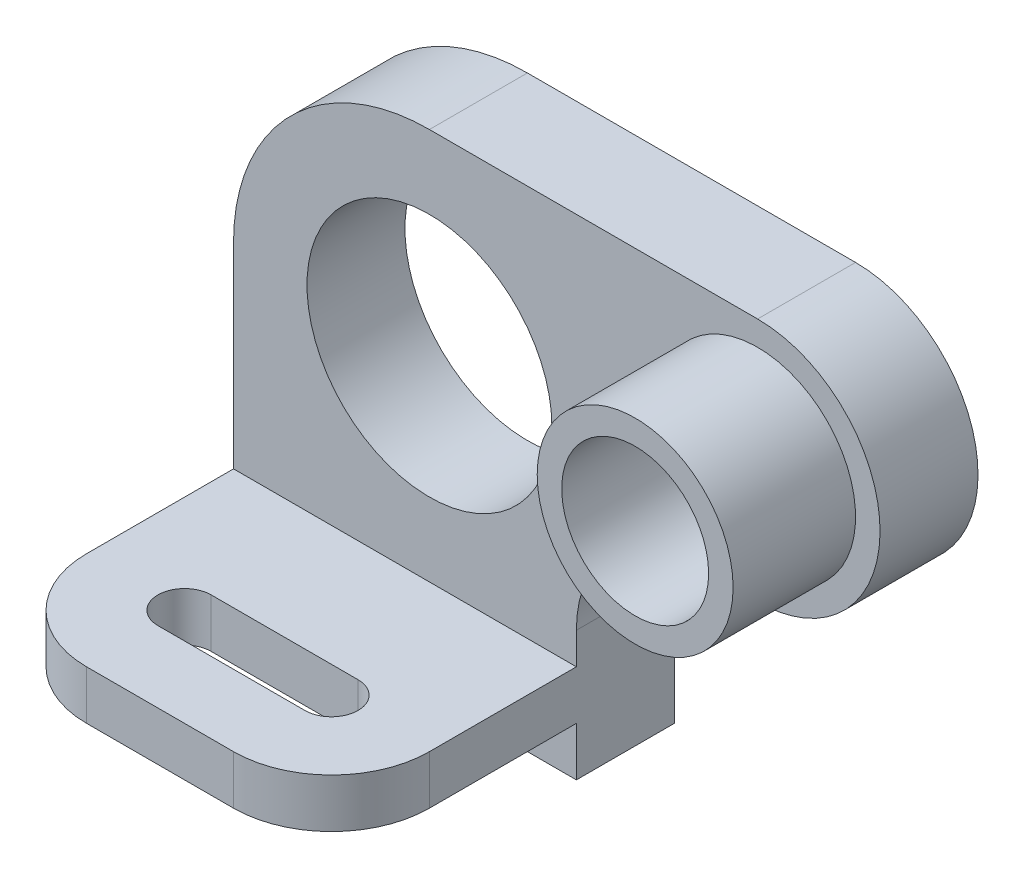
ISO-10303-21;
HEADER;
FILE_DESCRIPTION(('STEP AP214'),'2;1');
FILE_NAME('part.step','',(''),(''),'','','');
FILE_SCHEMA(('AUTOMOTIVE_DESIGN { 1 0 10303 214 1 1 1 1 }'));
ENDSEC;
DATA;
#1=APPLICATION_CONTEXT('core data for automotive mechanical design processes');
#2=APPLICATION_PROTOCOL_DEFINITION('international standard','automotive_design',2000,#1);
#3=PRODUCT_CONTEXT('',#1,'mechanical');
#4=PRODUCT('Part','Part','',(#3));
#5=PRODUCT_RELATED_PRODUCT_CATEGORY('part','',(#4));
#6=PRODUCT_DEFINITION_FORMATION('','',#4);
#7=PRODUCT_DEFINITION_CONTEXT('part definition',#1,'design');
#8=PRODUCT_DEFINITION('design','',#6,#7);
#9=PRODUCT_DEFINITION_SHAPE('','',#8);
#10=(LENGTH_UNIT() NAMED_UNIT(*) SI_UNIT(.MILLI.,.METRE.));
#11=(NAMED_UNIT(*) PLANE_ANGLE_UNIT() SI_UNIT($,.RADIAN.));
#12=(NAMED_UNIT(*) SI_UNIT($,.STERADIAN.) SOLID_ANGLE_UNIT());
#13=UNCERTAINTY_MEASURE_WITH_UNIT(LENGTH_MEASURE(1.E-05),#10,'distance_accuracy_value','');
#14=(GEOMETRIC_REPRESENTATION_CONTEXT(3) GLOBAL_UNCERTAINTY_ASSIGNED_CONTEXT((#13)) GLOBAL_UNIT_ASSIGNED_CONTEXT((#10,
#11,#12)) REPRESENTATION_CONTEXT('',''));
#15=CARTESIAN_POINT('',(0.,0.,0.));
#16=DIRECTION('',(0.,0.,1.));
#17=DIRECTION('',(1.,0.,0.));
#18=AXIS2_PLACEMENT_3D('',#15,#16,#17);
#19=CARTESIAN_POINT('',(40.,60.,20.));
#20=DIRECTION('',(0.,0.,-1.));
#21=DIRECTION('',(-1.,0.,0.));
#22=AXIS2_PLACEMENT_3D('',#19,#20,#21);
#23=PLANE('',#22);
#24=CARTESIAN_POINT('',(107.,75.,20.));
#25=DIRECTION('',(0.,0.,-1.));
#26=DIRECTION('',(-1.,0.,0.));
#27=AXIS2_PLACEMENT_3D('',#24,#25,#26);
#28=CIRCLE('',#27,20.);
#29=CARTESIAN_POINT('',(87.,75.,20.));
#30=VERTEX_POINT('',#29);
#31=EDGE_CURVE('E281',#30,#30,#28,.F.);
#32=ORIENTED_EDGE('',*,*,#31,.F.);
#33=EDGE_LOOP('',(#32));
#34=FACE_BOUND('',#33,.T.);
#35=CARTESIAN_POINT('',(40.,60.,20.));
#36=DIRECTION('',(0.,0.,1.));
#37=DIRECTION('',(1.,0.,0.));
#38=AXIS2_PLACEMENT_3D('',#35,#36,#37);
#39=CIRCLE('',#38,25.);
#40=CARTESIAN_POINT('',(65.,60.,20.));
#41=VERTEX_POINT('',#40);
#42=EDGE_CURVE('E215',#41,#41,#39,.T.);
#43=ORIENTED_EDGE('',*,*,#42,.F.);
#44=EDGE_LOOP('',(#43));
#45=FACE_BOUND('',#44,.T.);
#46=DIRECTION('',(-1.,0.,0.));
#47=VECTOR('',#46,1.);
#48=CARTESIAN_POINT('',(0.,20.,20.));
#49=LINE('',#48,#47);
#50=CARTESIAN_POINT('',(70.,20.,20.));
#51=VERTEX_POINT('',#50);
#52=CARTESIAN_POINT('',(0.,20.,20.));
#53=VERTEX_POINT('',#52);
#54=EDGE_CURVE('E190',#51,#53,#49,.T.);
#55=ORIENTED_EDGE('',*,*,#54,.F.);
#56=DIRECTION('',(0.,1.,0.));
#57=VECTOR('',#56,1.);
#58=CARTESIAN_POINT('',(70.,26.4613556019535,20.));
#59=LINE('',#58,#57);
#60=CARTESIAN_POINT('',(70.,26.4613556019535,20.));
#61=VERTEX_POINT('',#60);
#62=EDGE_CURVE('E232',#51,#61,#59,.T.);
#63=ORIENTED_EDGE('',*,*,#62,.T.);
#64=CARTESIAN_POINT('',(95.,26.4613556019535,20.));
#65=DIRECTION('',(0.,0.,-1.));
#66=DIRECTION('',(-1.,0.,0.));
#67=AXIS2_PLACEMENT_3D('',#64,#65,#66);
#68=CIRCLE('',#67,25.);
#69=CARTESIAN_POINT('',(101.,50.7306778009767,20.));
#70=VERTEX_POINT('',#69);
#71=EDGE_CURVE('E236',#61,#70,#68,.T.);
#72=ORIENTED_EDGE('',*,*,#71,.T.);
#73=CARTESIAN_POINT('',(107.,75.,20.));
#74=DIRECTION('',(0.,0.,1.));
#75=DIRECTION('',(1.,0.,0.));
#76=AXIS2_PLACEMENT_3D('',#73,#74,#75);
#77=CIRCLE('',#76,25.);
#78=CARTESIAN_POINT('',(107.,100.,20.));
#79=VERTEX_POINT('',#78);
#80=EDGE_CURVE('E238',#70,#79,#77,.T.);
#81=ORIENTED_EDGE('',*,*,#80,.T.);
#82=DIRECTION('',(-1.,0.,0.));
#83=VECTOR('',#82,1.);
#84=CARTESIAN_POINT('',(40.,100.,20.));
#85=LINE('',#84,#83);
#86=CARTESIAN_POINT('',(40.,100.,20.));
#87=VERTEX_POINT('',#86);
#88=EDGE_CURVE('E242',#79,#87,#85,.T.);
#89=ORIENTED_EDGE('',*,*,#88,.T.);
#90=CARTESIAN_POINT('',(40.,60.,20.));
#91=DIRECTION('',(0.,0.,1.));
#92=DIRECTION('',(-1.,0.,0.));
#93=AXIS2_PLACEMENT_3D('',#90,#91,#92);
#94=CIRCLE('',#93,40.);
#95=CARTESIAN_POINT('',(0.,60.,20.));
#96=VERTEX_POINT('',#95);
#97=EDGE_CURVE('E243',#87,#96,#94,.T.);
#98=ORIENTED_EDGE('',*,*,#97,.T.);
#99=DIRECTION('',(0.,-1.,0.));
#100=VECTOR('',#99,1.);
#101=CARTESIAN_POINT('',(0.,0.,20.));
#102=LINE('',#101,#100);
#103=EDGE_CURVE('E229',#96,#53,#102,.T.);
#104=ORIENTED_EDGE('',*,*,#103,.T.);
#105=EDGE_LOOP('',(#55,#63,#72,#81,#89,#98,#104));
#106=FACE_BOUND('',#105,.T.);
#107=ADVANCED_FACE('F44',(#34,#45,#106),#23,.F.);
#108=DIRECTION('',(1.,0.,0.));
#109=VECTOR('',#108,1.);
#110=CARTESIAN_POINT('',(0.,10.,20.));
#111=LINE('',#110,#109);
#112=CARTESIAN_POINT('',(0.,10.,20.));
#113=VERTEX_POINT('',#112);
#114=CARTESIAN_POINT('',(70.,10.,20.));
#115=VERTEX_POINT('',#114);
#116=EDGE_CURVE('E197',#113,#115,#111,.T.);
#117=ORIENTED_EDGE('',*,*,#116,.F.);
#118=CARTESIAN_POINT('',(0.,0.,20.));
#119=VERTEX_POINT('',#118);
#120=EDGE_CURVE('E235',#113,#119,#102,.T.);
#121=ORIENTED_EDGE('',*,*,#120,.T.);
#122=DIRECTION('',(1.,0.,0.));
#123=VECTOR('',#122,1.);
#124=CARTESIAN_POINT('',(0.,0.,20.));
#125=LINE('',#124,#123);
#126=CARTESIAN_POINT('',(70.,0.,20.));
#127=VERTEX_POINT('',#126);
#128=EDGE_CURVE('E231',#119,#127,#125,.T.);
#129=ORIENTED_EDGE('',*,*,#128,.T.);
#130=EDGE_CURVE('E234',#127,#115,#59,.T.);
#131=ORIENTED_EDGE('',*,*,#130,.T.);
#132=EDGE_LOOP('',(#117,#121,#129,#131));
#133=FACE_BOUND('',#132,.T.);
#134=ADVANCED_FACE('F324',(#133),#23,.F.);
#135=CARTESIAN_POINT('',(0.,0.,20.));
#136=DIRECTION('',(1.,0.,0.));
#137=DIRECTION('',(0.,0.,-1.));
#138=AXIS2_PLACEMENT_3D('',#135,#136,#137);
#139=PLANE('',#138);
#140=DIRECTION('',(0.,0.,-1.));
#141=VECTOR('',#140,1.);
#142=CARTESIAN_POINT('',(0.,10.,70.));
#143=LINE('',#142,#141);
#144=CARTESIAN_POINT('',(0.,10.,50.));
#145=VERTEX_POINT('',#144);
#146=EDGE_CURVE('E206',#145,#113,#143,.T.);
#147=ORIENTED_EDGE('',*,*,#146,.F.);
#148=DIRECTION('',(0.,-1.,0.));
#149=VECTOR('',#148,1.);
#150=CARTESIAN_POINT('',(0.,20.,50.));
#151=LINE('',#150,#149);
#152=CARTESIAN_POINT('',(0.,20.,50.));
#153=VERTEX_POINT('',#152);
#154=EDGE_CURVE('E294',#145,#153,#151,.F.);
#155=ORIENTED_EDGE('',*,*,#154,.T.);
#156=DIRECTION('',(0.,0.,-1.));
#157=VECTOR('',#156,1.);
#158=CARTESIAN_POINT('',(0.,20.,70.));
#159=LINE('',#158,#157);
#160=EDGE_CURVE('E208',#153,#53,#159,.T.);
#161=ORIENTED_EDGE('',*,*,#160,.T.);
#162=ORIENTED_EDGE('',*,*,#103,.F.);
#163=DIRECTION('',(0.,0.,-1.));
#164=VECTOR('',#163,1.);
#165=CARTESIAN_POINT('',(0.,60.,20.));
#166=LINE('',#165,#164);
#167=CARTESIAN_POINT('',(0.,60.,0.));
#168=VERTEX_POINT('',#167);
#169=EDGE_CURVE('E246',#96,#168,#166,.T.);
#170=ORIENTED_EDGE('',*,*,#169,.T.);
#171=DIRECTION('',(0.,-1.,0.));
#172=VECTOR('',#171,1.);
#173=CARTESIAN_POINT('',(0.,0.,0.));
#174=LINE('',#173,#172);
#175=CARTESIAN_POINT('',(0.,0.,0.));
#176=VERTEX_POINT('',#175);
#177=EDGE_CURVE('E227',#168,#176,#174,.T.);
#178=ORIENTED_EDGE('',*,*,#177,.T.);
#179=DIRECTION('',(0.,0.,-1.));
#180=VECTOR('',#179,1.);
#181=CARTESIAN_POINT('',(0.,0.,20.));
#182=LINE('',#181,#180);
#183=EDGE_CURVE('E279',#119,#176,#182,.T.);
#184=ORIENTED_EDGE('',*,*,#183,.F.);
#185=ORIENTED_EDGE('',*,*,#120,.F.);
#186=EDGE_LOOP('',(#147,#155,#161,#162,#170,#178,#184,#185));
#187=FACE_BOUND('',#186,.T.);
#188=ADVANCED_FACE('F335',(#187),#139,.F.);
#189=CARTESIAN_POINT('',(0.,0.,20.));
#190=DIRECTION('',(0.,1.,0.));
#191=DIRECTION('',(0.,0.,1.));
#192=AXIS2_PLACEMENT_3D('',#189,#190,#191);
#193=PLANE('',#192);
#194=DIRECTION('',(1.,0.,0.));
#195=VECTOR('',#194,1.);
#196=CARTESIAN_POINT('',(0.,0.,0.));
#197=LINE('',#196,#195);
#198=CARTESIAN_POINT('',(70.,0.,0.));
#199=VERTEX_POINT('',#198);
#200=EDGE_CURVE('E247',#176,#199,#197,.T.);
#201=ORIENTED_EDGE('',*,*,#200,.T.);
#202=DIRECTION('',(0.,0.,-1.));
#203=VECTOR('',#202,1.);
#204=CARTESIAN_POINT('',(70.,0.,20.));
#205=LINE('',#204,#203);
#206=EDGE_CURVE('E274',#127,#199,#205,.T.);
#207=ORIENTED_EDGE('',*,*,#206,.F.);
#208=ORIENTED_EDGE('',*,*,#128,.F.);
#209=ORIENTED_EDGE('',*,*,#183,.T.);
#210=EDGE_LOOP('',(#201,#207,#208,#209));
#211=FACE_BOUND('',#210,.T.);
#212=ADVANCED_FACE('F398',(#211),#193,.F.);
#213=CARTESIAN_POINT('',(70.,26.4613556019535,20.));
#214=DIRECTION('',(-1.,0.,0.));
#215=DIRECTION('',(0.,0.,1.));
#216=AXIS2_PLACEMENT_3D('',#213,#214,#215);
#217=PLANE('',#216);
#218=DIRECTION('',(0.,0.,-1.));
#219=VECTOR('',#218,1.);
#220=CARTESIAN_POINT('',(70.,20.,70.));
#221=LINE('',#220,#219);
#222=CARTESIAN_POINT('',(70.,20.,50.));
#223=VERTEX_POINT('',#222);
#224=EDGE_CURVE('E209',#223,#51,#221,.T.);
#225=ORIENTED_EDGE('',*,*,#224,.F.);
#226=DIRECTION('',(0.,1.,0.));
#227=VECTOR('',#226,1.);
#228=CARTESIAN_POINT('',(70.,10.,50.));
#229=LINE('',#228,#227);
#230=CARTESIAN_POINT('',(70.,10.,50.));
#231=VERTEX_POINT('',#230);
#232=EDGE_CURVE('E300',#223,#231,#229,.F.);
#233=ORIENTED_EDGE('',*,*,#232,.T.);
#234=DIRECTION('',(0.,0.,-1.));
#235=VECTOR('',#234,1.);
#236=CARTESIAN_POINT('',(70.,10.,70.));
#237=LINE('',#236,#235);
#238=EDGE_CURVE('E199',#231,#115,#237,.T.);
#239=ORIENTED_EDGE('',*,*,#238,.T.);
#240=ORIENTED_EDGE('',*,*,#130,.F.);
#241=ORIENTED_EDGE('',*,*,#206,.T.);
#242=DIRECTION('',(0.,1.,0.));
#243=VECTOR('',#242,1.);
#244=CARTESIAN_POINT('',(70.,26.4613556019535,0.));
#245=LINE('',#244,#243);
#246=CARTESIAN_POINT('',(70.,26.4613556019535,0.));
#247=VERTEX_POINT('',#246);
#248=EDGE_CURVE('E253',#199,#247,#245,.T.);
#249=ORIENTED_EDGE('',*,*,#248,.T.);
#250=DIRECTION('',(0.,0.,-1.));
#251=VECTOR('',#250,1.);
#252=CARTESIAN_POINT('',(70.,26.4613556019535,20.));
#253=LINE('',#252,#251);
#254=EDGE_CURVE('E275',#61,#247,#253,.T.);
#255=ORIENTED_EDGE('',*,*,#254,.F.);
#256=ORIENTED_EDGE('',*,*,#62,.F.);
#257=EDGE_LOOP('',(#225,#233,#239,#240,#241,#249,#255,#256));
#258=FACE_BOUND('',#257,.T.);
#259=ADVANCED_FACE('F393',(#258),#217,.F.);
#260=CARTESIAN_POINT('',(95.,26.4613556019535,20.));
#261=DIRECTION('',(0.,0.,-1.));
#262=DIRECTION('',(-1.,0.,0.));
#263=AXIS2_PLACEMENT_3D('',#260,#261,#262);
#264=CYLINDRICAL_SURFACE('',#263,25.);
#265=CARTESIAN_POINT('',(95.,26.4613556019535,0.));
#266=DIRECTION('',(0.,0.,-1.));
#267=DIRECTION('',(-1.,0.,0.));
#268=AXIS2_PLACEMENT_3D('',#265,#266,#267);
#269=CIRCLE('',#268,25.);
#270=CARTESIAN_POINT('',(101.,50.7306778009767,0.));
#271=VERTEX_POINT('',#270);
#272=EDGE_CURVE('E251',#247,#271,#269,.T.);
#273=ORIENTED_EDGE('',*,*,#272,.T.);
#274=DIRECTION('',(0.,0.,-1.));
#275=VECTOR('',#274,1.);
#276=CARTESIAN_POINT('',(101.,50.7306778009767,20.));
#277=LINE('',#276,#275);
#278=EDGE_CURVE('E267',#70,#271,#277,.T.);
#279=ORIENTED_EDGE('',*,*,#278,.F.);
#280=ORIENTED_EDGE('',*,*,#71,.F.);
#281=ORIENTED_EDGE('',*,*,#254,.T.);
#282=EDGE_LOOP('',(#273,#279,#280,#281));
#283=FACE_BOUND('',#282,.T.);
#284=ADVANCED_FACE('F388',(#283),#264,.F.);
#285=CARTESIAN_POINT('',(107.,75.,20.));
#286=DIRECTION('',(0.,0.,-1.));
#287=DIRECTION('',(-1.,0.,0.));
#288=AXIS2_PLACEMENT_3D('',#285,#286,#287);
#289=CYLINDRICAL_SURFACE('',#288,25.);
#290=CARTESIAN_POINT('',(107.,75.,0.));
#291=DIRECTION('',(0.,0.,1.));
#292=DIRECTION('',(1.,0.,0.));
#293=AXIS2_PLACEMENT_3D('',#290,#291,#292);
#294=CIRCLE('',#293,25.);
#295=CARTESIAN_POINT('',(107.,100.,0.));
#296=VERTEX_POINT('',#295);
#297=EDGE_CURVE('E254',#271,#296,#294,.T.);
#298=ORIENTED_EDGE('',*,*,#297,.T.);
#299=DIRECTION('',(0.,0.,-1.));
#300=VECTOR('',#299,1.);
#301=CARTESIAN_POINT('',(107.,100.,20.));
#302=LINE('',#301,#300);
#303=EDGE_CURVE('E266',#79,#296,#302,.T.);
#304=ORIENTED_EDGE('',*,*,#303,.F.);
#305=ORIENTED_EDGE('',*,*,#80,.F.);
#306=ORIENTED_EDGE('',*,*,#278,.T.);
#307=EDGE_LOOP('',(#298,#304,#305,#306));
#308=FACE_BOUND('',#307,.T.);
#309=ADVANCED_FACE('F387',(#308),#289,.T.);
#310=CARTESIAN_POINT('',(40.,100.,20.));
#311=DIRECTION('',(0.,-1.,0.));
#312=DIRECTION('',(1.,0.,0.));
#313=AXIS2_PLACEMENT_3D('',#310,#311,#312);
#314=PLANE('',#313);
#315=DIRECTION('',(-1.,0.,0.));
#316=VECTOR('',#315,1.);
#317=CARTESIAN_POINT('',(40.,100.,0.));
#318=LINE('',#317,#316);
#319=CARTESIAN_POINT('',(40.,100.,0.));
#320=VERTEX_POINT('',#319);
#321=EDGE_CURVE('E260',#296,#320,#318,.T.);
#322=ORIENTED_EDGE('',*,*,#321,.T.);
#323=DIRECTION('',(0.,0.,-1.));
#324=VECTOR('',#323,1.);
#325=CARTESIAN_POINT('',(40.,100.,20.));
#326=LINE('',#325,#324);
#327=EDGE_CURVE('E263',#87,#320,#326,.T.);
#328=ORIENTED_EDGE('',*,*,#327,.F.);
#329=ORIENTED_EDGE('',*,*,#88,.F.);
#330=ORIENTED_EDGE('',*,*,#303,.T.);
#331=EDGE_LOOP('',(#322,#328,#329,#330));
#332=FACE_BOUND('',#331,.T.);
#333=ADVANCED_FACE('F377',(#332),#314,.F.);
#334=CARTESIAN_POINT('',(40.,60.,20.));
#335=DIRECTION('',(0.,0.,-1.));
#336=DIRECTION('',(-1.,0.,0.));
#337=AXIS2_PLACEMENT_3D('',#334,#335,#336);
#338=CYLINDRICAL_SURFACE('',#337,40.);
#339=CARTESIAN_POINT('',(40.,60.,0.));
#340=DIRECTION('',(0.,0.,1.));
#341=DIRECTION('',(-1.,0.,0.));
#342=AXIS2_PLACEMENT_3D('',#339,#340,#341);
#343=CIRCLE('',#342,40.);
#344=EDGE_CURVE('E259',#320,#168,#343,.T.);
#345=ORIENTED_EDGE('',*,*,#344,.T.);
#346=ORIENTED_EDGE('',*,*,#169,.F.);
#347=ORIENTED_EDGE('',*,*,#97,.F.);
#348=ORIENTED_EDGE('',*,*,#327,.T.);
#349=EDGE_LOOP('',(#345,#346,#347,#348));
#350=FACE_BOUND('',#349,.T.);
#351=ADVANCED_FACE('F369',(#350),#338,.T.);
#352=CARTESIAN_POINT('',(40.,60.,0.));
#353=DIRECTION('',(0.,0.,-1.));
#354=DIRECTION('',(-1.,0.,0.));
#355=AXIS2_PLACEMENT_3D('',#352,#353,#354);
#356=PLANE('',#355);
#357=CARTESIAN_POINT('',(40.,60.,0.));
#358=DIRECTION('',(0.,0.,1.));
#359=DIRECTION('',(1.,0.,0.));
#360=AXIS2_PLACEMENT_3D('',#357,#358,#359);
#361=CIRCLE('',#360,25.);
#362=CARTESIAN_POINT('',(65.,60.,0.));
#363=VERTEX_POINT('',#362);
#364=EDGE_CURVE('E213',#363,#363,#361,.T.);
#365=ORIENTED_EDGE('',*,*,#364,.T.);
#366=EDGE_LOOP('',(#365));
#367=FACE_BOUND('',#366,.T.);
#368=ORIENTED_EDGE('',*,*,#177,.F.);
#369=ORIENTED_EDGE('',*,*,#344,.F.);
#370=ORIENTED_EDGE('',*,*,#321,.F.);
#371=ORIENTED_EDGE('',*,*,#297,.F.);
#372=ORIENTED_EDGE('',*,*,#272,.F.);
#373=ORIENTED_EDGE('',*,*,#248,.F.);
#374=ORIENTED_EDGE('',*,*,#200,.F.);
#375=EDGE_LOOP('',(#368,#369,#370,#371,#372,#373,#374));
#376=FACE_BOUND('',#375,.T.);
#377=ADVANCED_FACE('F361',(#367,#376),#356,.T.);
#378=CARTESIAN_POINT('',(107.,75.,45.));
#379=DIRECTION('',(0.,0.,1.));
#380=DIRECTION('',(1.,0.,0.));
#381=AXIS2_PLACEMENT_3D('',#378,#379,#380);
#382=PLANE('',#381);
#383=CARTESIAN_POINT('',(107.,75.,45.));
#384=DIRECTION('',(0.,0.,1.));
#385=DIRECTION('',(1.,0.,0.));
#386=AXIS2_PLACEMENT_3D('',#383,#384,#385);
#387=CIRCLE('',#386,20.);
#388=CARTESIAN_POINT('',(127.,75.,45.));
#389=VERTEX_POINT('',#388);
#390=EDGE_CURVE('E225',#389,#389,#387,.T.);
#391=ORIENTED_EDGE('',*,*,#390,.T.);
#392=EDGE_LOOP('',(#391));
#393=FACE_BOUND('',#392,.T.);
#394=CARTESIAN_POINT('',(107.,75.,45.));
#395=DIRECTION('',(0.,0.,1.));
#396=DIRECTION('',(1.,0.,0.));
#397=AXIS2_PLACEMENT_3D('',#394,#395,#396);
#398=CIRCLE('',#397,15.);
#399=CARTESIAN_POINT('',(122.,75.,45.));
#400=VERTEX_POINT('',#399);
#401=EDGE_CURVE('E218',#400,#400,#398,.T.);
#402=ORIENTED_EDGE('',*,*,#401,.F.);
#403=EDGE_LOOP('',(#402));
#404=FACE_BOUND('',#403,.T.);
#405=ADVANCED_FACE('F358',(#393,#404),#382,.T.);
#406=CARTESIAN_POINT('',(107.,75.,45.));
#407=DIRECTION('',(0.,0.,-1.));
#408=DIRECTION('',(-1.,0.,0.));
#409=AXIS2_PLACEMENT_3D('',#406,#407,#408);
#410=CYLINDRICAL_SURFACE('',#409,20.);
#411=ORIENTED_EDGE('',*,*,#390,.F.);
#412=EDGE_LOOP('',(#411));
#413=FACE_BOUND('',#412,.T.);
#414=ORIENTED_EDGE('',*,*,#31,.T.);
#415=EDGE_LOOP('',(#414));
#416=FACE_BOUND('',#415,.T.);
#417=ADVANCED_FACE('F348',(#413,#416),#410,.T.);
#418=CARTESIAN_POINT('',(107.,75.,45.));
#419=DIRECTION('',(0.,0.,-1.));
#420=DIRECTION('',(-1.,0.,0.));
#421=AXIS2_PLACEMENT_3D('',#418,#419,#420);
#422=CYLINDRICAL_SURFACE('',#421,15.);
#423=ORIENTED_EDGE('',*,*,#401,.T.);
#424=EDGE_LOOP('',(#423));
#425=FACE_BOUND('',#424,.T.);
#426=CARTESIAN_POINT('',(107.,75.,20.));
#427=DIRECTION('',(0.,0.,1.));
#428=DIRECTION('',(1.,0.,0.));
#429=AXIS2_PLACEMENT_3D('',#426,#427,#428);
#430=CIRCLE('',#429,15.);
#431=CARTESIAN_POINT('',(122.,75.,20.));
#432=VERTEX_POINT('',#431);
#433=EDGE_CURVE('E216',#432,#432,#430,.T.);
#434=ORIENTED_EDGE('',*,*,#433,.F.);
#435=EDGE_LOOP('',(#434));
#436=FACE_BOUND('',#435,.T.);
#437=ADVANCED_FACE('F340',(#425,#436),#422,.F.);
#438=ORIENTED_EDGE('',*,*,#433,.T.);
#439=EDGE_LOOP('',(#438));
#440=FACE_BOUND('',#439,.T.);
#441=ADVANCED_FACE('F327',(#440),#23,.F.);
#442=CARTESIAN_POINT('',(40.,60.,0.));
#443=DIRECTION('',(0.,0.,1.));
#444=DIRECTION('',(1.,0.,0.));
#445=AXIS2_PLACEMENT_3D('',#442,#443,#444);
#446=CYLINDRICAL_SURFACE('',#445,25.);
#447=ORIENTED_EDGE('',*,*,#364,.F.);
#448=EDGE_LOOP('',(#447));
#449=FACE_BOUND('',#448,.T.);
#450=ORIENTED_EDGE('',*,*,#42,.T.);
#451=EDGE_LOOP('',(#450));
#452=FACE_BOUND('',#451,.T.);
#453=ADVANCED_FACE('F338',(#449,#452),#446,.F.);
#454=CARTESIAN_POINT('',(0.,20.,70.));
#455=DIRECTION('',(0.,-1.,0.));
#456=DIRECTION('',(0.,0.,-1.));
#457=AXIS2_PLACEMENT_3D('',#454,#455,#456);
#458=PLANE('',#457);
#459=DIRECTION('',(1.,0.,0.));
#460=VECTOR('',#459,1.);
#461=CARTESIAN_POINT('',(20.,20.,55.4352905579183));
#462=LINE('',#461,#460);
#463=CARTESIAN_POINT('',(20.,20.,55.4352905579183));
#464=VERTEX_POINT('',#463);
#465=CARTESIAN_POINT('',(50.,20.,55.4352905579183));
#466=VERTEX_POINT('',#465);
#467=EDGE_CURVE('E176',#464,#466,#462,.T.);
#468=ORIENTED_EDGE('',*,*,#467,.F.);
#469=CARTESIAN_POINT('',(20.,20.,50.));
#470=DIRECTION('',(0.,1.,0.));
#471=DIRECTION('',(0.,0.,1.));
#472=AXIS2_PLACEMENT_3D('',#469,#470,#471);
#473=CIRCLE('',#472,5.43529055791828);
#474=CARTESIAN_POINT('',(20.,20.,44.5647094420817));
#475=VERTEX_POINT('',#474);
#476=EDGE_CURVE('E58',#475,#464,#473,.T.);
#477=ORIENTED_EDGE('',*,*,#476,.F.);
#478=DIRECTION('',(-1.,0.,0.));
#479=VECTOR('',#478,1.);
#480=CARTESIAN_POINT('',(20.,20.,44.5647094420817));
#481=LINE('',#480,#479);
#482=CARTESIAN_POINT('',(50.,20.,44.5647094420817));
#483=VERTEX_POINT('',#482);
#484=EDGE_CURVE('E181',#483,#475,#481,.T.);
#485=ORIENTED_EDGE('',*,*,#484,.F.);
#486=CARTESIAN_POINT('',(50.,20.,50.));
#487=DIRECTION('',(0.,1.,0.));
#488=DIRECTION('',(0.,0.,1.));
#489=AXIS2_PLACEMENT_3D('',#486,#487,#488);
#490=CIRCLE('',#489,5.43529055791828);
#491=EDGE_CURVE('E170',#466,#483,#490,.T.);
#492=ORIENTED_EDGE('',*,*,#491,.F.);
#493=EDGE_LOOP('',(#468,#477,#485,#492));
#494=FACE_BOUND('',#493,.T.);
#495=ORIENTED_EDGE('',*,*,#160,.F.);
#496=CARTESIAN_POINT('',(20.,20.,50.));
#497=DIRECTION('',(0.,-1.,0.));
#498=DIRECTION('',(0.,0.,-1.));
#499=AXIS2_PLACEMENT_3D('',#496,#497,#498);
#500=CIRCLE('',#499,20.);
#501=CARTESIAN_POINT('',(20.,20.,70.));
#502=VERTEX_POINT('',#501);
#503=EDGE_CURVE('E299',#153,#502,#500,.F.);
#504=ORIENTED_EDGE('',*,*,#503,.T.);
#505=DIRECTION('',(-1.,0.,0.));
#506=VECTOR('',#505,1.);
#507=CARTESIAN_POINT('',(0.,20.,70.));
#508=LINE('',#507,#506);
#509=CARTESIAN_POINT('',(50.,20.,70.));
#510=VERTEX_POINT('',#509);
#511=EDGE_CURVE('E193',#510,#502,#508,.T.);
#512=ORIENTED_EDGE('',*,*,#511,.F.);
#513=CARTESIAN_POINT('',(50.,20.,50.));
#514=DIRECTION('',(0.,-1.,0.));
#515=DIRECTION('',(0.,0.,-1.));
#516=AXIS2_PLACEMENT_3D('',#513,#514,#515);
#517=CIRCLE('',#516,20.);
#518=EDGE_CURVE('E296',#510,#223,#517,.F.);
#519=ORIENTED_EDGE('',*,*,#518,.T.);
#520=ORIENTED_EDGE('',*,*,#224,.T.);
#521=ORIENTED_EDGE('',*,*,#54,.T.);
#522=EDGE_LOOP('',(#495,#504,#512,#519,#520,#521));
#523=FACE_BOUND('',#522,.T.);
#524=ADVANCED_FACE('F179',(#494,#523),#458,.F.);
#525=CARTESIAN_POINT('',(0.,10.,70.));
#526=DIRECTION('',(0.,1.,0.));
#527=DIRECTION('',(0.,0.,1.));
#528=AXIS2_PLACEMENT_3D('',#525,#526,#527);
#529=PLANE('',#528);
#530=DIRECTION('',(-1.,0.,0.));
#531=VECTOR('',#530,1.);
#532=CARTESIAN_POINT('',(0.,10.,44.5647094420817));
#533=LINE('',#532,#531);
#534=CARTESIAN_POINT('',(50.,10.,44.5647094420817));
#535=VERTEX_POINT('',#534);
#536=CARTESIAN_POINT('',(20.,10.,44.5647094420817));
#537=VERTEX_POINT('',#536);
#538=EDGE_CURVE('E52',#535,#537,#533,.T.);
#539=ORIENTED_EDGE('',*,*,#538,.T.);
#540=CARTESIAN_POINT('',(20.,10.,50.));
#541=DIRECTION('',(0.,1.,0.));
#542=DIRECTION('',(0.,0.,1.));
#543=AXIS2_PLACEMENT_3D('',#540,#541,#542);
#544=CIRCLE('',#543,5.43529055791828);
#545=CARTESIAN_POINT('',(20.,10.,55.4352905579183));
#546=VERTEX_POINT('',#545);
#547=EDGE_CURVE('E11',#537,#546,#544,.T.);
#548=ORIENTED_EDGE('',*,*,#547,.T.);
#549=DIRECTION('',(1.,0.,0.));
#550=VECTOR('',#549,1.);
#551=CARTESIAN_POINT('',(0.,10.,55.4352905579183));
#552=LINE('',#551,#550);
#553=CARTESIAN_POINT('',(50.,10.,55.4352905579183));
#554=VERTEX_POINT('',#553);
#555=EDGE_CURVE('E305',#546,#554,#552,.T.);
#556=ORIENTED_EDGE('',*,*,#555,.T.);
#557=CARTESIAN_POINT('',(50.,10.,50.));
#558=DIRECTION('',(0.,1.,0.));
#559=DIRECTION('',(0.,0.,1.));
#560=AXIS2_PLACEMENT_3D('',#557,#558,#559);
#561=CIRCLE('',#560,5.43529055791828);
#562=EDGE_CURVE('E168',#554,#535,#561,.T.);
#563=ORIENTED_EDGE('',*,*,#562,.T.);
#564=EDGE_LOOP('',(#539,#548,#556,#563));
#565=FACE_BOUND('',#564,.T.);
#566=DIRECTION('',(1.,0.,0.));
#567=VECTOR('',#566,1.);
#568=CARTESIAN_POINT('',(0.,10.,70.));
#569=LINE('',#568,#567);
#570=CARTESIAN_POINT('',(20.,10.,70.));
#571=VERTEX_POINT('',#570);
#572=CARTESIAN_POINT('',(50.,10.,70.));
#573=VERTEX_POINT('',#572);
#574=EDGE_CURVE('E198',#571,#573,#569,.T.);
#575=ORIENTED_EDGE('',*,*,#574,.F.);
#576=CARTESIAN_POINT('',(20.,10.,50.));
#577=DIRECTION('',(0.,1.,0.));
#578=DIRECTION('',(0.,0.,1.));
#579=AXIS2_PLACEMENT_3D('',#576,#577,#578);
#580=CIRCLE('',#579,20.);
#581=EDGE_CURVE('E295',#571,#145,#580,.F.);
#582=ORIENTED_EDGE('',*,*,#581,.T.);
#583=ORIENTED_EDGE('',*,*,#146,.T.);
#584=ORIENTED_EDGE('',*,*,#116,.T.);
#585=ORIENTED_EDGE('',*,*,#238,.F.);
#586=CARTESIAN_POINT('',(50.,10.,50.));
#587=DIRECTION('',(0.,1.,0.));
#588=DIRECTION('',(0.,0.,1.));
#589=AXIS2_PLACEMENT_3D('',#586,#587,#588);
#590=CIRCLE('',#589,20.);
#591=EDGE_CURVE('E289',#231,#573,#590,.F.);
#592=ORIENTED_EDGE('',*,*,#591,.T.);
#593=EDGE_LOOP('',(#575,#582,#583,#584,#585,#592));
#594=FACE_BOUND('',#593,.T.);
#595=ADVANCED_FACE('F308',(#565,#594),#529,.F.);
#596=CARTESIAN_POINT('',(0.,0.,70.));
#597=DIRECTION('',(0.,0.,1.));
#598=DIRECTION('',(1.,0.,0.));
#599=AXIS2_PLACEMENT_3D('',#596,#597,#598);
#600=PLANE('',#599);
#601=ORIENTED_EDGE('',*,*,#511,.T.);
#602=DIRECTION('',(0.,-1.,0.));
#603=VECTOR('',#602,1.);
#604=CARTESIAN_POINT('',(20.,10.,70.));
#605=LINE('',#604,#603);
#606=EDGE_CURVE('E290',#502,#571,#605,.T.);
#607=ORIENTED_EDGE('',*,*,#606,.T.);
#608=ORIENTED_EDGE('',*,*,#574,.T.);
#609=DIRECTION('',(0.,1.,0.));
#610=VECTOR('',#609,1.);
#611=CARTESIAN_POINT('',(50.,20.,70.));
#612=LINE('',#611,#610);
#613=EDGE_CURVE('E283',#573,#510,#612,.T.);
#614=ORIENTED_EDGE('',*,*,#613,.T.);
#615=EDGE_LOOP('',(#601,#607,#608,#614));
#616=FACE_BOUND('',#615,.T.);
#617=ADVANCED_FACE('F406',(#616),#600,.T.);
#618=CARTESIAN_POINT('',(20.,0.,50.));
#619=DIRECTION('',(0.,1.,0.));
#620=DIRECTION('',(0.,0.,1.));
#621=AXIS2_PLACEMENT_3D('',#618,#619,#620);
#622=CYLINDRICAL_SURFACE('',#621,20.);
#623=ORIENTED_EDGE('',*,*,#503,.F.);
#624=ORIENTED_EDGE('',*,*,#154,.F.);
#625=ORIENTED_EDGE('',*,*,#581,.F.);
#626=ORIENTED_EDGE('',*,*,#606,.F.);
#627=EDGE_LOOP('',(#623,#624,#625,#626));
#628=FACE_BOUND('',#627,.T.);
#629=ADVANCED_FACE('F319',(#628),#622,.T.);
#630=CARTESIAN_POINT('',(50.,0.,50.));
#631=DIRECTION('',(0.,-1.,0.));
#632=DIRECTION('',(0.,0.,-1.));
#633=AXIS2_PLACEMENT_3D('',#630,#631,#632);
#634=CYLINDRICAL_SURFACE('',#633,20.);
#635=ORIENTED_EDGE('',*,*,#591,.F.);
#636=ORIENTED_EDGE('',*,*,#232,.F.);
#637=ORIENTED_EDGE('',*,*,#518,.F.);
#638=ORIENTED_EDGE('',*,*,#613,.F.);
#639=EDGE_LOOP('',(#635,#636,#637,#638));
#640=FACE_BOUND('',#639,.T.);
#641=ADVANCED_FACE('F50',(#640),#634,.T.);
#642=CARTESIAN_POINT('',(20.,0.,50.));
#643=DIRECTION('',(0.,1.,0.));
#644=DIRECTION('',(0.,0.,1.));
#645=AXIS2_PLACEMENT_3D('',#642,#643,#644);
#646=CYLINDRICAL_SURFACE('',#645,5.43529055791828);
#647=DIRECTION('',(0.,1.,0.));
#648=VECTOR('',#647,1.);
#649=CARTESIAN_POINT('',(20.,0.,44.5647094420817));
#650=LINE('',#649,#648);
#651=EDGE_CURVE('E189',#537,#475,#650,.T.);
#652=ORIENTED_EDGE('',*,*,#651,.T.);
#653=ORIENTED_EDGE('',*,*,#476,.T.);
#654=DIRECTION('',(0.,1.,0.));
#655=VECTOR('',#654,1.);
#656=CARTESIAN_POINT('',(20.,0.,55.4352905579183));
#657=LINE('',#656,#655);
#658=EDGE_CURVE('E174',#546,#464,#657,.T.);
#659=ORIENTED_EDGE('',*,*,#658,.F.);
#660=ORIENTED_EDGE('',*,*,#547,.F.);
#661=EDGE_LOOP('',(#652,#653,#659,#660));
#662=FACE_BOUND('',#661,.T.);
#663=ADVANCED_FACE('F313',(#662),#646,.F.);
#664=CARTESIAN_POINT('',(20.,0.,44.5647094420817));
#665=DIRECTION('',(0.,0.,-1.));
#666=DIRECTION('',(-1.,0.,0.));
#667=AXIS2_PLACEMENT_3D('',#664,#665,#666);
#668=PLANE('',#667);
#669=DIRECTION('',(0.,1.,0.));
#670=VECTOR('',#669,1.);
#671=CARTESIAN_POINT('',(50.,0.,44.5647094420817));
#672=LINE('',#671,#670);
#673=EDGE_CURVE('E172',#535,#483,#672,.T.);
#674=ORIENTED_EDGE('',*,*,#673,.T.);
#675=ORIENTED_EDGE('',*,*,#484,.T.);
#676=ORIENTED_EDGE('',*,*,#651,.F.);
#677=ORIENTED_EDGE('',*,*,#538,.F.);
#678=EDGE_LOOP('',(#674,#675,#676,#677));
#679=FACE_BOUND('',#678,.T.);
#680=ADVANCED_FACE('F309',(#679),#668,.F.);
#681=CARTESIAN_POINT('',(50.,0.,50.));
#682=DIRECTION('',(0.,1.,0.));
#683=DIRECTION('',(0.,0.,1.));
#684=AXIS2_PLACEMENT_3D('',#681,#682,#683);
#685=CYLINDRICAL_SURFACE('',#684,5.43529055791828);
#686=DIRECTION('',(0.,1.,0.));
#687=VECTOR('',#686,1.);
#688=CARTESIAN_POINT('',(50.,0.,55.4352905579183));
#689=LINE('',#688,#687);
#690=EDGE_CURVE('E68',#554,#466,#689,.T.);
#691=ORIENTED_EDGE('',*,*,#690,.T.);
#692=ORIENTED_EDGE('',*,*,#491,.T.);
#693=ORIENTED_EDGE('',*,*,#673,.F.);
#694=ORIENTED_EDGE('',*,*,#562,.F.);
#695=EDGE_LOOP('',(#691,#692,#693,#694));
#696=FACE_BOUND('',#695,.T.);
#697=ADVANCED_FACE('F163',(#696),#685,.F.);
#698=CARTESIAN_POINT('',(20.,0.,55.4352905579183));
#699=DIRECTION('',(0.,0.,1.));
#700=DIRECTION('',(1.,0.,0.));
#701=AXIS2_PLACEMENT_3D('',#698,#699,#700);
#702=PLANE('',#701);
#703=ORIENTED_EDGE('',*,*,#658,.T.);
#704=ORIENTED_EDGE('',*,*,#467,.T.);
#705=ORIENTED_EDGE('',*,*,#690,.F.);
#706=ORIENTED_EDGE('',*,*,#555,.F.);
#707=EDGE_LOOP('',(#703,#704,#705,#706));
#708=FACE_BOUND('',#707,.T.);
#709=ADVANCED_FACE('F180',(#708),#702,.F.);
#710=CLOSED_SHELL('',(#107,#134,#188,#212,#259,#284,#309,#333,#351,#377,#405,#417,#437,#441,
#453,#524,#595,#617,#629,#641,#663,#680,#697,#709));
#711=MANIFOLD_SOLID_BREP('B2',#710);
#712=ADVANCED_BREP_SHAPE_REPRESENTATION('',(#18,#711),#14);
#713=SHAPE_DEFINITION_REPRESENTATION(#9,#712);
ENDSEC;
END-ISO-10303-21;
